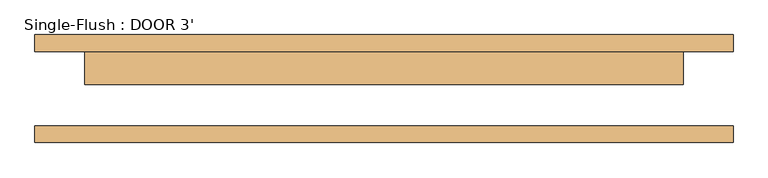
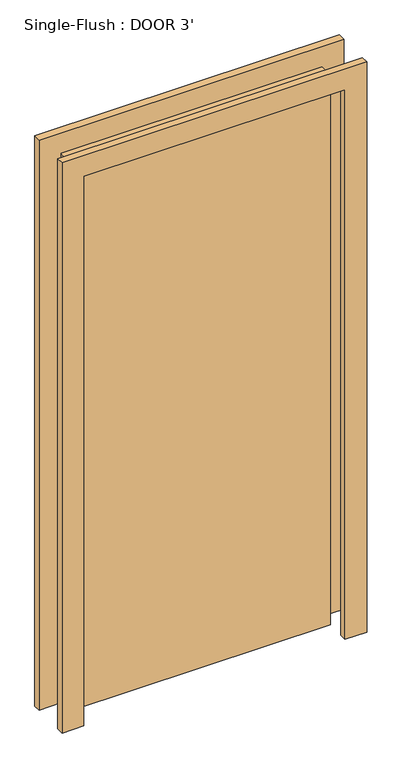
"""IFC4 building model written with IfcOpenShell, lengths in millimetres: door geometry, Single-Flush : DOOR 3'."""

from ifc_helpers import new_model, si_unit, frame, origin, origin_with_axes, place, context, project, spatial, polyline, outline, extrude, source, transform, mapped, element, save


def single_flush_door_3_17d80c48(model_context):
    return source(origin(), model_context, "Body", "SweptSolid", [
        extrude(outline(polyline([(2108.2, -533.4), (0.0, -533.4), (0.0, -457.2), (2032.0, -457.2), (2032.0, 457.2), (0.0, 457.2), (0.0, 533.4), (2108.2, 533.4), (2108.2, -533.4)])), frame((0.0, 57.15, 0.0), z_axis=(0.0, 1.0, 0.0), x_axis=(0.0, 0.0, 1.0)), (0.0, 0.0, 1.0), 25.4),
        extrude(outline(polyline([(2108.2, 533.4), (2108.2, -533.4), (0.0, -533.4), (0.0, -457.2), (2032.0, -457.2), (2032.0, 457.2), (0.0, 457.2), (0.0, 533.4), (2108.2, 533.4)])), frame((0.0, -82.55, 0.0), z_axis=(0.0, 1.0, 0.0), x_axis=(0.0, 0.0, 1.0)), (0.0, 0.0, 1.0), 25.4),
        extrude(outline(polyline([(457.2, 6.35), (-457.2, 6.35), (-457.2, 57.15), (457.2, 57.15), (457.2, 6.35)])), origin_with_axes(), (0.0, 0.0, 1.0), 2032.0),
    ])


if __name__ == "__main__":
    model = new_model("IFC4")
    model_context = context("Model", 3, world=origin())
    ifc_project = project(units=[si_unit("LENGTHUNIT", "METRE", prefix="MILLI")], contexts=[model_context])
    site = spatial("IfcSite", under=ifc_project)
    building = spatial("IfcBuilding", under=site)
    placement = place(None, origin())
    single_flush_door_3_shape = single_flush_door_3_17d80c48(model_context)
    element("IfcDoor", 1, ObjectType="Single-Flush : DOOR 3'", at=placement, inside=building, context=model_context, shape_type="MappedRepresentation", body=[
        mapped(single_flush_door_3_shape, transform((0.0, 0.0, 0.0), x_axis=(1.0, 0.0, 0.0), y_axis=(0.0, 1.0, 0.0), z_axis=(0.0, 0.0, 1.0))),
    ])
    save(model, "model.ifc")

# Revit data of these elements
# Type "Single-Flush : DOOR 3'"
#   Type Mark = "8"
#   Construction Type Id = "MDOOR"
#   Assembly Code = "C1020"
#   Analytic Construction = "Metal"
#   Thickness = 0' - 2"
#   Heat Transfer Coefficient (U) = 0.651978 BTU/(h·ft²·°F)
#   Height = 6' - 8"
#   Trim Projection Ext = 0' - 1"
#   Trim Projection Int = 0' - 1"
#   Trim Width = 0' - 3"
#   Width = 3' - 0"
#   Define Thermal Properties by = 1
#   Door Material = Door - Panel
#   Frame Material = Door - Frame
#   Visual Light Transmittance = 0
#   Solar Heat Gain Coefficient = 0
#   Function = (empty or 0)
#   Wall Closure = (empty or 0)
# Element 1 (IfcDoor, "Single-Flush : DOOR 3'")
#   Materials on its faces: "Door - Frame", "Door - Panel"
# Materials
#   "Door - Panel": class "Wood", colour RGB 210 159 95, transparency 0, Cost = 0
#   "Door - Frame": colour RGB 118 70 51, transparency 0, Cost = 0
